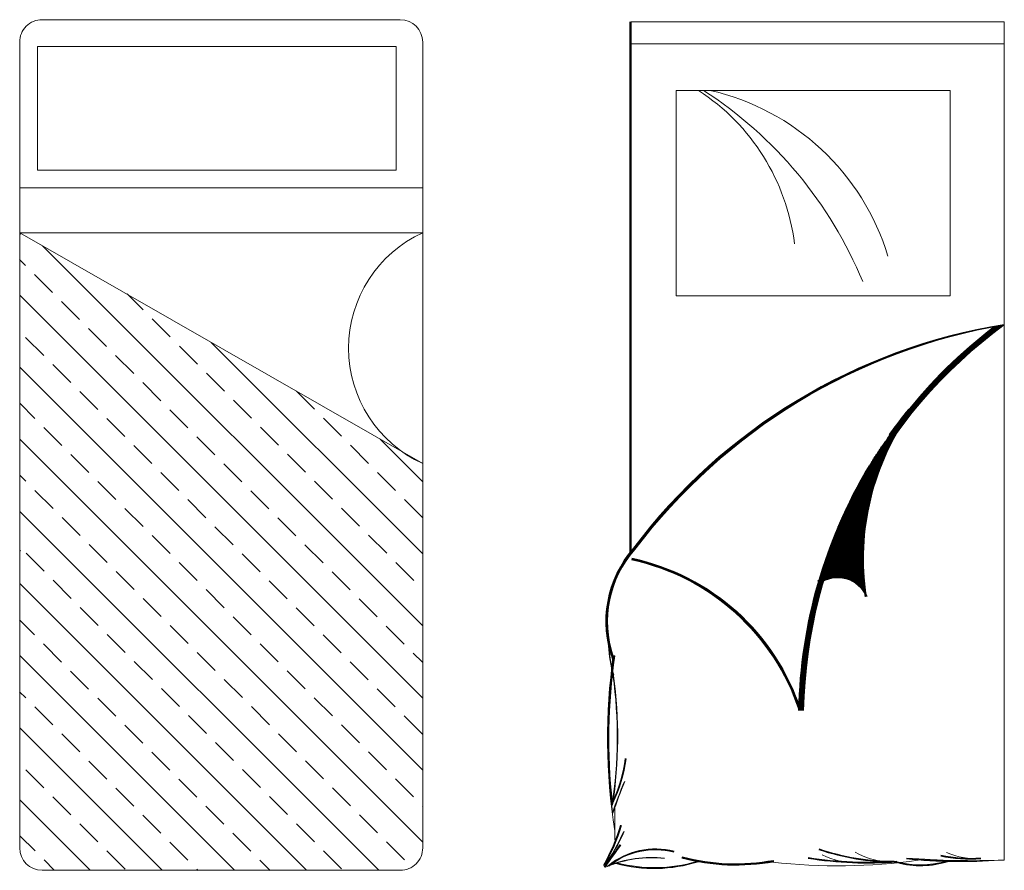
# Model space of a CAD drawing. Units: inches. Extents: x 1994 to 3075, y 3517 to 3950.
# Tile 16 of 58: x 1994.56064 to 1994.65565, y 3553.23331 to 3553.31541. Entities that reach past the tile are written whole.
import ezdxf

# ---------------------------------------------------------------- set-up
doc = ezdxf.new("R2010")
doc.units = ezdxf.units.IN
doc.layers.add('A-FURN-REFR', color=8, linetype='Continuous', lineweight=13)
doc.layers.add('A-FURN-REFR-PATT', color=8, linetype='Continuous', lineweight=13)

msp = doc.modelspace()

# ---------------------------------------------------------------- hatches: boundary and pattern name
at = {"layer": 'A-FURN-REFR-PATT'}
h = msp.add_hatch(dxfattribs=at)
h.set_pattern_fill('ANSI33', color=256, scale=0.0196850393700788, angle=90, style=0)
h.set_pattern_definition([(135, (2001.281701362167, 3543.018306419075), (-0.0034798562066267, -0.0034798562066267), []), (135, (2001.281701362167, 3543.021786275275), (-0.0034798562066267, -0.0034798562066267), [0.0024606299212598, -0.0012303149606299])])
h.paths.add_polyline_path([(1994.560750643588, 3553.294785964831), (1994.560641735829, 3553.294677057073), (1994.560641735829, 3553.235467034077, 0.4142135623730951), (1994.56280228893, 3553.233306480976), (1994.597371138556, 3553.233306480976, 0.4142135623732468), (1994.599531691658, 3553.235467034077), (1994.599531691658, 3553.272565954262, -0.0451375875559221), (1994.597615359404, 3553.273663937041)])

# ---------------------------------------------------------------- linework, layer by layer
at = {"layer": 'A-FURN-REFR'}
for p, q in [((1994.597371138556, 3553.315407498837), (1994.562802288931, 3553.315407498837)), ((1994.619511402385, 3553.315190146324), (1994.619511402385, 3553.263955990339)), ((1994.619555455342, 3553.315190146324), (1994.619555455342, 3553.264011295154)), ((1994.619599508299, 3553.315190146324), (1994.619599508299, 3553.264065859234)), ((1994.619599508299, 3553.315190146324), (1994.619599508299, 3553.264065859234)), ((1994.619599508299, 3553.315190146324), (1994.619599508299, 3553.264065859234)), ((1994.655654330193, 3553.315190146324), (1994.619599508299, 3553.315190146324)), ((1994.619643561256, 3553.315190146324), (1994.619643561256, 3553.264119700406)), ((1994.619643561256, 3553.315190146324), (1994.619643561256, 3553.264119700406)), ((1994.655654330193, 3553.315190146324), (1994.655654330193, 3553.234294758865)), ((1994.560641735829, 3553.313246945735), (1994.560641735829, 3553.235467034077)), ((1994.596955789959, 3553.31280465389), (1994.562373625505, 3553.312804653891)), ((1994.562373625505, 3553.312804653891), (1994.562373625505, 3553.300872194913)), ((1994.596955789959, 3553.300872194913), (1994.596955789959, 3553.31280465389)), ((1994.599531691658, 3553.235467034077), (1994.599531691658, 3553.313246945735)), ((1994.655654330193, 3553.313071196984), (1994.619599508299, 3553.313071196984)), ((1994.624004803977, 3553.308582202807), (1994.624004803977, 3553.288758372255)), ((1994.650436578046, 3553.308582202807), (1994.624004803977, 3553.308582202807)), ((1994.650436578046, 3553.308582202807), (1994.650436578046, 3553.288758372255)), ((1994.562373625505, 3553.300872194913), (1994.596955789959, 3553.300872194913)), ((1994.560641735829, 3553.299169470883), (1994.599531691658, 3553.299169470883)), ((1994.560641735829, 3553.29484836468), (1994.599531691658, 3553.29484836468)), ((1994.599531691658, 3553.272565954262), (1994.560641735829, 3553.29484836468)), ((1994.560641735829, 3553.294677057073), (1994.560750643588, 3553.294785964831)), ((1994.650436578046, 3553.288758372255), (1994.624004803977, 3553.288758372255)), ((1994.560641735829, 3553.264122222087), (1994.560732437507, 3553.264212923765)), ((1994.617837390028, 3553.25368698014), (1994.617837390028, 3553.252219708717)), ((1994.618073426563, 3553.239364958644), (1994.618073426563, 3553.236258299635)), ((1994.56280228893, 3553.233306480976), (1994.597371138556, 3553.233306480976))]:
    msp.add_line(p, q, dxfattribs=at)
for centre, radius, start, end in [((1994.562802288931, 3553.313246945735), 0.0021605531015945, 89.99999999966911, 180), ((1994.597371138556, 3553.313246945735), 0.0021605531015945, 0, 89.99999999966911), ((1994.614801182076, 3553.291181506897), 0.0207749763658571, 7.206665032643007, 56.88540460250624), ((1994.604826660356, 3553.274823269209), 0.0401896231626752, 22.38812789457889, 57.13920038385841), ((1994.622100128715, 3553.285843750796), 0.023313025712657, 16.76586877918271, 77.25302279903774), ((1994.60464244617, 3553.283707159472), 0.0122574983256972, 114.6421290173532, 245.3578709847273), ((1994.664529009929, 3553.230869281651), 0.0558368955091939, 99.14533752577712, 143.1101086982114), ((1994.664562076667, 3553.230840174026), 0.0558368955091939, 99.17970674840424, 143.1101086982114), ((1994.664771181835, 3553.230590799417), 0.0561102118056199, 99.35094038266166, 143.044287962684), ((1994.664988334941, 3553.230345836472), 0.0563869958724091, 99.52829798959606, 142.9784067690825), ((1994.665207821662, 3553.230098239676), 0.0566673036217349, 99.70579827647545, 142.9124677267231), ((1994.683580006847, 3553.247782049873), 0.0476515933188419, 127.0467796499212, 178.8543501141797), ((1994.683580006847, 3553.247782049873), 0.04760754036206, 126.9406482463485, 178.8543501141797), ((1994.683580006847, 3553.247782049873), 0.0475634874052781, 126.8343885346346, 178.8543501141797), ((1994.683580006847, 3553.247782049873), 0.0475194344484962, 126.7279997707044, 178.8543501141797), ((1994.683580006847, 3553.247782049873), 0.0474753814917143, 126.6214812070186, 178.8543501141797), ((1994.683580006847, 3553.247782049873), 0.0474313285349324, 126.5148320908192, 178.8543501141797), ((1994.683580006847, 3553.247782049873), 0.0473872755781505, 126.4080516645007, 178.8543501141797), ((1994.683580006847, 3553.247782049873), 0.0473432226213686, 126.3011391675447, 178.8543501141797), ((1994.683580006847, 3553.247782049873), 0.0472991696645867, 126.1940938326673, 178.8543501141797), ((1994.683580006847, 3553.247782049873), 0.0476956462756238, 127.1527834845398, 145.1946706884665), ((1994.683580006847, 3553.247782049873), 0.0477396992324057, 127.2586604854645, 141.8830102971661), ((1994.683580006847, 3553.247782049873), 0.0476956462756238, 127.4194857530354, 178.8543501141797), ((1994.683580006847, 3553.247782049873), 0.0473432226213686, 127.0578299505718, 178.8543501141797), ((1994.666461608342, 3553.263385325071), 0.024743608776698, 145.8476054945275, 186.7725521007765), ((1994.666461608342, 3553.263385325071), 0.0246995558199161, 145.8511400476067, 186.9337656671545), ((1994.666461608342, 3553.263385325071), 0.0246555028631342, 143.9610008614225, 187.1069136909233), ((1994.666461608342, 3553.263385325071), 0.0246114499063523, 143.9610008614225, 187.2941254414202), ((1994.666461608342, 3553.263385325071), 0.0245673969495704, 143.9610008614225, 187.4983101912694), ((1994.666461608342, 3553.263385325071), 0.0245233439927885, 143.9610008614225, 188.6168638438873), ((1994.666461608342, 3553.263385325071), 0.0244792910360066, 143.9610008614225, 187.9764444592905), ((1994.666461608342, 3553.263385325071), 0.0244352380792247, 143.9610008614225, 188.6168638438873), ((1994.666461608342, 3553.263385325071), 0.0243911851224427, 143.9610008614225, 188.6168638438873), ((1994.683580006847, 3553.247782049873), 0.0477396992324057, 141.0347968380583, 145.1979078254653), ((1994.683580006847, 3553.247782049873), 0.0477837521891876, 141.0362621045667, 144.7543200533534), ((1994.666461608342, 3553.263385325071), 0.0248317146902618, 148.3932359561964, 186.4798219117168), ((1994.666461608342, 3553.263385325071), 0.0247876617334799, 147.2064653698421, 186.6216577350586), ((1994.683580006847, 3553.247782049873), 0.0477396992324057, 142.5889521864169, 145.1979078254653), ((1994.666461608342, 3553.263385325071), 0.0249198206038257, 150.4366277158946, 186.2194853925298), ((1994.666461608342, 3553.263385325071), 0.0248757676470437, 149.4599240533851, 186.3460377258838), ((1994.683580006847, 3553.247782049873), 0.0477396992324057, 145.6204067247484, 178.8543501141797), ((1994.683580006847, 3553.247782049873), 0.0476956462756238, 145.6169941061015, 178.8543501141797), ((1994.666461608342, 3553.263385325071), 0.0250519794741714, 153.7583543314393, 185.876959704691), ((1994.666461608342, 3553.263385325071), 0.0250079265173895, 152.9982327015039, 185.9854724011842), ((1994.666461608342, 3553.263385325071), 0.0249638735606076, 152.1973192474915, 186.0994866187383), ((1994.666461608342, 3553.263385325071), 0.0252722442580809, 156.4781873319089, 185.4041716682919), ((1994.666461608342, 3553.263385325071), 0.025228191301299, 155.8362227067639, 185.4904151679532), ((1994.666461608342, 3553.263385325071), 0.0251841383445171, 155.169838355571, 185.5805559357272), ((1994.666461608342, 3553.263385325071), 0.0251400853877352, 154.4761275716599, 185.6748372652484), ((1994.666461608342, 3553.263385325071), 0.0250960324309533, 154.4832169162481, 185.7735342056219), ((1994.666461608342, 3553.263385325071), 0.0254484560852086, 158.8450917996622, 185.0941654085052), ((1994.666461608342, 3553.263385325071), 0.0254044031284267, 158.2799831538903, 185.1667713232256), ((1994.666461608342, 3553.263385325071), 0.0253603501716447, 157.6981722127393, 185.242533517558), ((1994.666461608342, 3553.263385325071), 0.0253603501716447, 157.6981722127393, 185.242533517558), ((1994.666461608342, 3553.263385325071), 0.0253162972148628, 157.0981553803312, 185.3216089806067), ((1994.666461608342, 3553.263385325071), 0.0253162972148628, 157.0981553803312, 185.3216089806067), ((1994.683580006847, 3553.247782049873), 0.0477837521891876, 149.0499074590062, 178.8543501141797), ((1994.683580006847, 3553.247782049873), 0.0477396992324057, 149.045120457143, 178.8543501141797), ((1994.666461608342, 3553.263385325071), 0.0256687208691181, 161.4606583605357, 184.773922266981), ((1994.666461608342, 3553.263385325071), 0.0256246679123362, 160.9623463509966, 184.832644249888), ((1994.666461608342, 3553.263385325071), 0.0255806149555543, 160.4524808872289, 184.8939259311579), ((1994.666461608342, 3553.263385325071), 0.0255365619987724, 159.9302648881264, 184.9578663729609), ((1994.666461608342, 3553.263385325071), 0.0254925090419905, 159.3948045088843, 185.0245735359543), ((1994.666461608342, 3553.263385325071), 0.0258889856530277, 163.8016215093118, 184.5157526806098), ((1994.666461608342, 3553.263385325071), 0.0258449326962457, 163.3516489443423, 184.562911180991), ((1994.666461608342, 3553.263385325071), 0.0258008797394638, 162.8930716875973, 184.612238069312), ((1994.666461608342, 3553.263385325071), 0.0257568267826819, 162.4254085226018, 184.6638000036539), ((1994.666461608342, 3553.263385325071), 0.0257127738259, 161.9481313217683, 184.7176688583396), ((1994.666461608342, 3553.263385325071), 0.0261092504369372, 165.9366187090828, 184.31046215666), ((1994.666461608342, 3553.263385325071), 0.0260651974801553, 165.5237411763672, 184.3476266088035), ((1994.666461608342, 3553.263385325071), 0.0260211445233734, 165.1041324353788, 184.3866894669623), ((1994.666461608342, 3553.263385325071), 0.0259770915665915, 164.677475931831, 184.4276974607441), ((1994.666461608342, 3553.263385325071), 0.0259770915665915, 164.677475931831, 184.4276974607441), ((1994.666461608342, 3553.263385325071), 0.0259330386098096, 164.2434293392044, 184.4707006433081), ((1994.666461608342, 3553.263385325071), 0.0263735681776287, 168.2876097026887, 184.1250834940751), ((1994.666461608342, 3553.263385325071), 0.0263295152208468, 167.9096203257427, 184.151682375002), ((1994.666461608342, 3553.263385325071), 0.0262854622640648, 167.5263849310796, 184.1799562386341), ((1994.666461608342, 3553.263385325071), 0.0262414093072829, 167.1376962784207, 184.2099364825078), ((1994.666461608342, 3553.263385325071), 0.026197356350501, 166.7433330500798, 184.2416566222153), ((1994.666461608342, 3553.263385325071), 0.0261533033937191, 166.3430584635889, 184.2751524406097), ((1994.666461608342, 3553.263385325071), 0.0266378859183201, 170.4554940936222, 183.9991417037784), ((1994.666461608342, 3553.263385325071), 0.0265938329615382, 170.1052781174558, 184.016247045014), ((1994.666461608342, 3553.263385325071), 0.0265497800047563, 169.7508241457858, 184.0348766875957), ((1994.666461608342, 3553.263385325071), 0.0265057270479744, 169.3919877760861, 184.0550517619501), ((1994.666461608342, 3553.263385325071), 0.0264616740911925, 169.0286161897971, 184.0767948713113), ((1994.666461608342, 3553.263385325071), 0.0264176211344106, 168.6605474476658, 184.1001301789581), ((1994.666461608342, 3553.263385325071), 0.0269462566157935, 172.7989734885977, 183.9205884776596), ((1994.666461608342, 3553.263385325071), 0.0269022036590116, 172.474967087972, 183.9275053389765), ((1994.666461608342, 3553.263385325071), 0.0268581507022297, 172.1475446049654, 183.9358344844096), ((1994.666461608342, 3553.263385325071), 0.0268140977454478, 171.8166056543932, 183.9455884404993), ((1994.666461608342, 3553.263385325071), 0.0267700447886659, 171.4820448324587, 183.9567808171263), ((1994.666461608342, 3553.263385325071), 0.0267259918318839, 171.1437513634359, 183.9694263478359), ((1994.666461608342, 3553.263385325071), 0.026681938875102, 170.8016087000953, 183.983540936691), ((1994.666461608342, 3553.263385325071), 0.0272105743564849, 174.6763415735681, 183.9081723278276), ((1994.666461608342, 3553.263385325071), 0.0272105743564849, 174.6763415735681, 183.9081723278276), ((1994.666461608342, 3553.263385325071), 0.027166521399703, 174.3709660785187, 183.9068217927131), ((1994.666461608342, 3553.263385325071), 0.0271224684429211, 174.0626881956943, 183.9068294357355), ((1994.666461608342, 3553.263385325071), 0.0270784154861392, 173.7514315741923, 183.9082018903319), ((1994.666461608342, 3553.263385325071), 0.0270343625293573, 173.4371164660456, 183.9109467180485), ((1994.666461608342, 3553.263385325071), 0.0269903095725754, 173.1196595086898, 183.9150724238507), ((1994.666461608342, 3553.263385325071), 0.0272546273132668, 174.978887833532, 183.9108753176306), ((1994.627902683089, 3553.257317127372), 0.0106999109031217, 138.6435372436876, 200.3899182151953), ((1994.627902683089, 3553.257317127372), 0.0106558579463398, 138.6435372436876, 199.9442973805121), ((1994.627902683089, 3553.257317127372), 0.0106118049895579, 138.6435372436876, 199.4900821614752), ((1994.627902683089, 3553.257317127372), 0.010567752032776, 138.6435372436876, 199.0268875545775), ((1994.627902683089, 3553.257317127372), 0.0105236990759941, 138.6435372436876, 198.5542988813752), ((1994.639584966185, 3553.258533765415), 0.0053880087456002, 62.5281077128473, 100.8579597591114), ((1994.639584966185, 3553.258533765415), 0.0054320617023821, 62.77055770140147, 100.5845671939894), ((1994.639584966185, 3553.258533765415), 0.0054761146591641, 63.0074083270334, 100.3156564957506), ((1994.615127727357, 3553.241936055818), 0.0218070014713327, 18.13038786915423, 77.93345558165026), ((1994.615127727357, 3553.241936055818), 0.0218510544281146, 18.13038786915423, 77.93345558165026), ((1994.615127727357, 3553.241936055818), 0.0218510544281146, 18.13038786915423, 77.93345558165026), ((1994.615127727357, 3553.241936055818), 0.0218951073848965, 18.13038786915423, 77.93345558165026), ((1994.615127727357, 3553.241936055818), 0.0219391603416785, 18.13038786915423, 77.93345558165026), ((1994.615127727357, 3553.241936055818), 0.0219832132984604, 18.13038786915423, 77.93345558165026), ((1994.639584966185, 3553.258533765415), 0.0044188436963982, 55.29409319829883, 108.3503866603046), ((1994.639584966185, 3553.258533765415), 0.0044628966531801, 55.72689734416534, 107.9313424196028), ((1994.639584966185, 3553.258533765415), 0.0045069496099621, 56.14688551534506, 107.5216800677553), ((1994.639584966185, 3553.258533765415), 0.004551002566744, 56.55462986218708, 107.1210395469069), ((1994.639584966185, 3553.258533765415), 0.0045950555235259, 56.95066501292508, 106.7290803815871), ((1994.639584966185, 3553.258533765415), 0.0046391084803078, 57.33549138251529, 106.345480275258), ((1994.639584966185, 3553.258533765415), 0.0046831614370897, 57.70957811356919, 105.9699338357063), ((1994.639584966185, 3553.258533765415), 0.0047272143938716, 58.07336570302371, 105.6021514081261), ((1994.639584966185, 3553.258533765415), 0.0047712673506535, 58.42726834486711, 105.2418580111888), ((1994.639584966185, 3553.258533765415), 0.0048153203074354, 58.77167603508624, 104.8887923629696), ((1994.639584966185, 3553.258533765415), 0.0048593732642173, 59.10695646164525, 104.5427059866208), ((1994.639584966185, 3553.258533765415), 0.0049034262209992, 59.43345671342008, 104.2033623878335), ((1994.639584966185, 3553.258533765415), 0.0049474791777811, 59.75150481685821, 103.8705363009669), ((1994.639584966185, 3553.258533765415), 0.0049915321345631, 60.06141113529348, 103.5440129922504), ((1994.639584966185, 3553.258533765415), 0.005035585091345, 60.36346963390639, 103.2235876162559), ((1994.639584966185, 3553.258533765415), 0.0050796380481269, 60.65795903444319, 102.9090646223622), ((1994.639584966185, 3553.258533765415), 0.0050796380481269, 60.65795903444319, 102.9090646223622), ((1994.639584966185, 3553.258533765415), 0.0051236910049088, 60.94514386415502, 102.6002572061999), ((1994.639584966185, 3553.258533765415), 0.0051236910049088, 60.94514386415502, 102.6002572061999), ((1994.639584966185, 3553.258533765415), 0.0051236910049088, 60.94514386415502, 102.6002572061999), ((1994.639584966185, 3553.258533765415), 0.0051677439616907, 61.22527541734137, 102.2969867995423), ((1994.639584966185, 3553.258533765415), 0.0052117969184726, 61.49859263164885, 101.9990825971519), ((1994.639584966185, 3553.258533765415), 0.0052558498752545, 61.76532289556114, 101.7063811210097), ((1994.639584966185, 3553.258533765415), 0.0052999028320364, 62.02568278469914, 101.41872580812), ((1994.639584966185, 3553.258533765415), 0.0053439557888183, 62.27987874420942, 101.1359666347343), ((1994.639584966185, 3553.258533765415), 0.0034937316039781, 41.4702865128866, 120.2885680207145), ((1994.639584966185, 3553.258533765415), 0.00353778456076, 42.45556402315891, 119.5269216475722), ((1994.639584966185, 3553.258533765415), 0.003581837517542, 43.3892877521526, 118.7921509098936), ((1994.639584966185, 3553.258533765415), 0.0036258904743239, 44.2763908618006, 118.0825630294143), ((1994.639584966185, 3553.258533765415), 0.0036699434311058, 45.1210753821295, 117.3966238194631), ((1994.639584966185, 3553.258533765415), 0.0037139963878877, 45.92695739005882, 116.7329377061916), ((1994.639584966185, 3553.258533765415), 0.0037580493446696, 46.69717680231321, 116.0902308985833), ((1994.639584966185, 3553.258533765415), 0.0038021023014515, 47.43448182913776, 115.4673371165979), ((1994.639584966185, 3553.258533765415), 0.0038461552582334, 48.14129491839708, 114.8631854132095), ((1994.639584966185, 3553.258533765415), 0.0038902082150153, 48.81976494417092, 114.2767897258904), ((1994.639584966185, 3553.258533765415), 0.0039342611717972, 49.47180901428468, 113.7072398626937), ((1994.639584966185, 3553.258533765415), 0.0039783141285791, 50.09914632093672, 113.1536936892395), ((1994.639584966185, 3553.258533765415), 0.004022367085361, 50.70332582884353, 112.6153703254441), ((1994.639584966185, 3553.258533765415), 0.004066420042143, 51.2857491220135, 112.0915441934747), ((1994.639584966185, 3553.258533765415), 0.0041104729989249, 51.84768941428586, 111.5815397929198), ((1994.639584966185, 3553.258533765415), 0.0041545259557068, 52.39030748711694, 111.0847270942413), ((1994.639584966185, 3553.258533765415), 0.0041985789124887, 52.91466514686622, 110.600517464643), ((1994.639584966185, 3553.258533765415), 0.0041985789124887, 52.91466514686622, 110.600517464643), ((1994.639584966185, 3553.258533765415), 0.0042426318692706, 53.42173665687948, 110.1283600498166), ((1994.639584966185, 3553.258533765415), 0.0042866848260525, 53.91241851272671, 109.6677385542701), ((1994.639584966185, 3553.258533765415), 0.0043307377828344, 54.38753784247719, 109.218168364243), ((1994.639584966185, 3553.258533765415), 0.0043747907396163, 54.84785966646155, 108.7791939721919), ((1994.639584966185, 3553.258533765415), 0.0033175197768505, 36.87602587035403, 126.0120691195208), ((1994.639584966185, 3553.258533765415), 0.0032294138632867, 34.03685203068306, 126.0120691195208), ((1994.639584966185, 3553.258533765415), 0.0031853609065048, 32.41922698042424, 126.0120691195208), ((1994.639584966185, 3553.258533765415), 0.0032734668200686, 35.51426843498751, 124.5737538345291), ((1994.639584966185, 3553.258533765415), 0.0031413079497229, 30.62639575645341, 126.0120691195208), ((1994.639584966185, 3553.258533765415), 0.003097254992941, 23.44233100441356, 126.0120691195208), ((1994.639584966185, 3553.258533765415), 0.0033615727336324, 38.14016662308291, 122.7546046628128), ((1994.639584966185, 3553.258533765415), 0.0034056256904143, 39.32043347813337, 121.9001999235671), ((1994.639584966185, 3553.258533765415), 0.003053202036159, 23.44233100441356, 126.0120691195208), ((1994.639584966185, 3553.258533765415), 0.0034496786471962, 40.42759520581463, 121.0789652796015), ((1994.639584966185, 3553.258533765415), 0.0030091490793771, 23.44233100441356, 126.0120691195208), ((1994.630130448194, 3553.255647219901), 0.0126866289837311, 183.0211004818441, 196.0160169042029), ((1994.630130448194, 3553.255647219901), 0.0126425760269492, 184.1845599757889, 196.0160169042029), ((1994.673580722078, 3553.246028811499), 0.0562182202085284, 171.8072076161304, 189.1215704248215), ((1994.673580722078, 3553.246028811499), 0.0561741672517465, 171.8072076161304, 187.3008679287846), ((1994.673580722078, 3553.246028811499), 0.0561301142949646, 171.8072076161304, 186.5176513869889), ((1994.673580722078, 3553.246028811499), 0.0560860613381827, 171.8072076161304, 186.2948159241982), ((1994.575361267159, 3553.246149578681), 0.0429456485675089, 351.2257733735594, 7.968227192195032), ((1994.575361267159, 3553.246149578681), 0.0429897015242908, 351.2257733735594, 7.968227192195032), ((1994.604483159655, 3553.246122351538), 0.014825439053331, 334.6763726611908, 352.0716805907631), ((1994.604483159655, 3553.246122351538), 0.0147813860965491, 335.1483445702522, 352.0716805907631), ((1994.604483159655, 3553.246122351538), 0.0147373331397672, 335.7324461056919, 352.0716805907631), ((1994.66631529492, 3553.222343504094), 0.0512007512239989, 157.5594257430853, 161.1924953734588), ((1994.66631529492, 3553.222343504094), 0.051156698267217, 157.5594257430853, 161.1924953734588), ((1994.599941623127, 3553.243376303709), 0.0195457880346728, 330.6769944071866, 342.9761611028538), ((1994.599941623127, 3553.243376303709), 0.0195898409914547, 330.6769944071866, 342.9761611028538), ((1994.599941623127, 3553.243376303709), 0.0196338939482367, 330.6769944071866, 342.9761611028538), ((1994.599835627817, 3553.245517275303), 0.0208834327279857, 325.6693661681979, 336.093599378745), ((1994.599835627817, 3553.245517275303), 0.0209274856847676, 325.6693661681979, 336.093599378745), ((1994.56280228893, 3553.235467034077), 0.0021605531015945, 180, 269.9999999996691), ((1994.597371138556, 3553.235467034077), 0.0021605531015945, 269.9999999996691, 0), ((1994.666295370655, 3553.20006118261), 0.0596097442102864, 143.1616544898542, 145.7225303623336), ((1994.666295370655, 3553.20006118261), 0.0595656912535045, 143.1616544898542, 145.7225303623336), ((1994.666295370655, 3553.20006118261), 0.0595216382967226, 143.1616544898542, 145.7225303623336), ((1994.621625843466, 3553.223124430301), 0.0114337521600424, 83.7956822385169, 112.3575152583951), ((1994.621625843466, 3553.223124430301), 0.0113896992032605, 83.7956822385169, 112.3575152583951), ((1994.621999281649, 3553.228064312342), 0.0073088492151716, 75.85795039232165, 128.4689099467231), ((1994.621999281649, 3553.228064312342), 0.0072647962583897, 75.85795039232165, 128.4689099467231), ((1994.621999281649, 3553.228064312342), 0.0072207433016078, 75.85795039232165, 128.4689099467231), ((1994.629746983706, 3553.253804897391), 0.0200051988196854, 254.8913445911323, 280.5672360393155), ((1994.629746983706, 3553.253804897391), 0.0199611458629035, 254.8913445911323, 280.5672360393155), ((1994.629746983706, 3553.253804897391), 0.0199170929061216, 254.8913445911323, 280.5672360393155), ((1994.629746983706, 3553.253804897391), 0.0198730399493397, 254.8913445911323, 280.5672360393155), ((1994.642564000497, 3553.272230622579), 0.0381890973478346, 261.203467349764, 274.0922678359194), ((1994.642564000497, 3553.272230622579), 0.0381450443910527, 261.203467349764, 274.0922678359194), ((1994.645014881928, 3553.256750006206), 0.0226550596903131, 251.356587876115, 270.0346240651407), ((1994.645014881928, 3553.256750006206), 0.0226110067335312, 251.356587876115, 270.0346240651407), ((1994.645014881928, 3553.256750006206), 0.0225669537767493, 251.356587876115, 270.0346240651407), ((1994.641451091062, 3553.24156434986), 0.0075581635227854, 243.5148083386907, 270.7838517998538), ((1994.645149414539, 3553.242090726108), 0.0080381684178949, 240.9529325713119, 264.1129596014716), ((1994.652603363444, 3553.314514863708), 0.0802781017418674, 265.4384925031771, 272.1780488464221), ((1994.652438487106, 3553.249029862782), 0.0146572330658983, 258.4912000779365, 273.698481814418), ((1994.652438487106, 3553.249029862782), 0.0146131801091164, 258.4912000779365, 273.698481814418), ((1994.652438487106, 3553.249029862782), 0.0145691271523344, 258.4912000779365, 273.698481814418), ((1994.652898383926, 3553.241437819568), 0.007007479444016, 246.3360717811442, 273.9734741061417), ((1994.621872320652, 3553.247601460731), 0.0141287021381247, 254.732529968135, 287.5373657651138), ((1994.621872320652, 3553.247601460731), 0.0140846491813428, 255.0114324104398, 287.1997291768062), ((1994.621872320652, 3553.247601460731), 0.0140405962245609, 255.2988484411373, 286.8600482220965), ((1994.639627635492, 3553.289498718291), 0.0557657762709106, 263.4679660053708, 277.966072432154), ((1994.642564000497, 3553.272230622579), 0.0382331503046165, 261.203467349764, 274.0922678359194), ((1994.647590790739, 3553.242422777343), 0.008681614899649, 254.6485408536564, 287.9402315840665), ((1994.647590790739, 3553.242422777343), 0.008637561942867, 254.6485408536564, 287.0864281475689), ((1994.647590790739, 3553.242422777343), 0.0085935089860851, 254.6485408536564, 286.191156545447), ((1994.651473284374, 3553.288923394467), 0.0547734476607441, 264.4886281806342, 273.956506610001), ((1994.651931664435, 3553.299313537746), 0.065117787808889, 264.9642351938961, 272.923297310608)]:
    msp.add_arc(centre, radius, start, end, dxfattribs=at)

doc.saveas('drawing.dxf')
